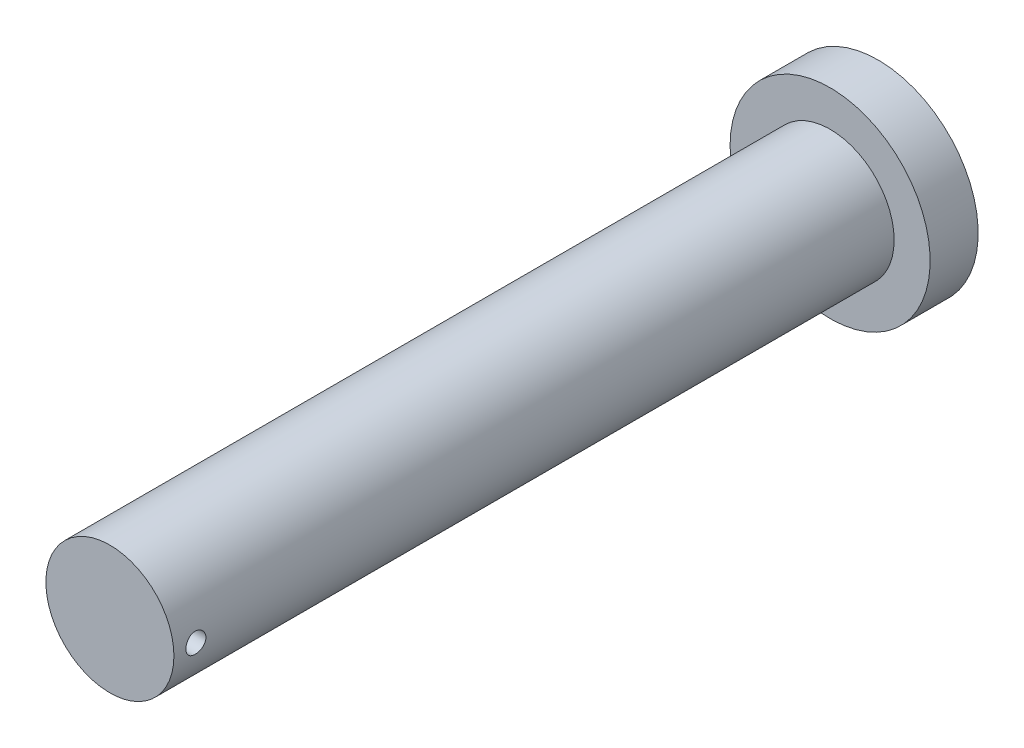
SolidWorks part; units mm, degrees
material "Plain Carbon Steel"
ref_plane "Front Plane" through (0, 0, 0) normal (0, 0, 1) x (1, 0, 0)
ref_plane "Top Plane" through (0, 0, 0) normal (0, 1, 0) x (1, 0, 0)
ref_plane "Right Plane" through (0, 0, 0) normal (1, 0, 0) x (0, 0, -1)
sketch "Shank Profile Ø32" plane through (0, 0, 0) normal (0, 0, 1) x (1, 0, 0)
  circle A0 centre (0, 0) radius 16
  dimension "D1" = 32
extrude "Shank Ø32x180" add sketch "Shank Profile Ø32" along normal blind 180
sketch "Head Profile Ø50" plane through (0, 0, 0) normal (0, 0, -1) x (-1, 0, 0)
  circle A0 centre (0, 0) radius 25
  dimension "D1" = 50
extrude "Head Ø50x12" add sketch "Head Profile Ø50" along normal blind 12
sketch "Cross Hole Profile Ø5" plane through (0, 0, 0) normal (1, 0, 0) x (0, 0, -1)
  line L0 (-180, 16) -> (-180, -16) construction
  circle A0 centre (-174.5, 0) radius 2.5
  dimension "D1" = 5
  dimension "D2" = 5.5
  dimension "D3" = 174.5
extrude "Cross Hole Ø5" cut sketch "Cross Hole Profile Ø5" against normal mid plane 150
